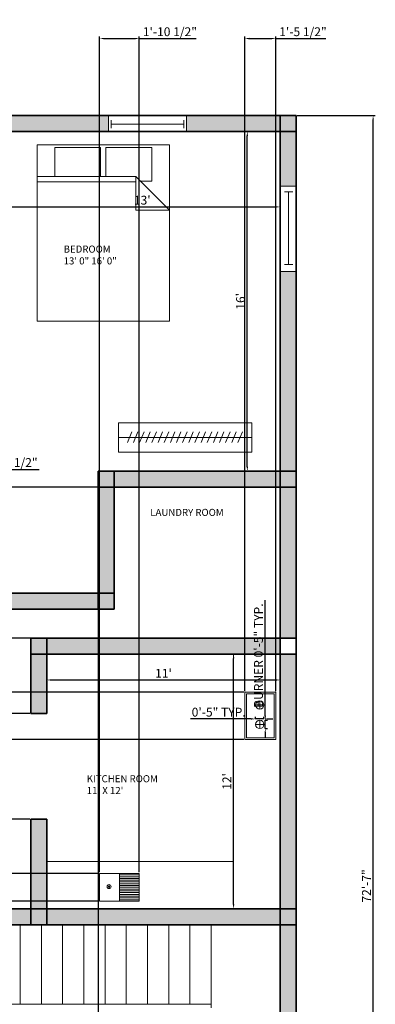
# Model space of a CAD drawing. Units: millimetres. Extents: x 2936 to 3516, y 349 to 1320.
# Tile 5 of 5: x 3315 to 3516, y 763 to 1320. Entities that reach past the tile are written whole.
import ezdxf

# ---------------------------------------------------------------- set-up
doc = ezdxf.new("R2010")
doc.units = ezdxf.units.MM
for name, color, linetype, lineweight in [('A-ANNO-DIMS', 3, 'Continuous', 13), ('A-AREA-IDEN', 190, 'Continuous', 18), ('A-EQPM', 140, 'Continuous', 18), ('A-FLOR-CASE', 140, 'Continuous', 18), ('A-FLOR-CASE-PATT', 140, 'Continuous', 13), ('A-FLOR-FIXT', 140, 'Continuous', 18), ('A-FLOR-FIXT-PATT', 140, 'Continuous', 13), ('A-WALL-PATT', 50, 'Continuous', 13), ('furniture', 140, 'Continuous', 18), ('staircase', 170, 'Continuous', 18), ('walls', 50, 'Continuous', 35), ('windows', 30, 'Continuous', 18)]:
    doc.layers.add(name, color=color, linetype=linetype, lineweight=lineweight)
doc.styles.get("Standard").update_dxf_attribs({"font": 'arial.ttf'})
doc.dimstyles.new('ISO-25', dxfattribs={"dimtxt": 5, "dimasz": 2.5, "dimexe": 1.25, "dimexo": 0.625, "dimtad": 1, "dimdec": 0, "dimlunit": 3, "dimtxsty": 'Standard', "dimcen": 2.5, "dimadec": 0, "dimazin": 0, "dimtfac": 1, "dimtdec": 0, "dimtmove": 0, "dimatfit": 3, "dimfxl": 1, "dimarcsym": 0})

# ---------------------------------------------------------------- blocks, each defined once
blk = doc.blocks.new('*U4')
for p, q in [((0, 4), (0, 0)), ((0, 2), (36, 2)), ((36, 4), (36, 0))]:
    blk.add_line(p, q)
blk = doc.blocks.new('Bed - Queen')
for p, q in [((0, -80.00003), (0, 0)), ((0, 0), (59.99999, 0)), ((59.99999, 0), (59.99999, -80.00003)), ((7.99999, -1.2), (28.79998, -1.2)), ((7.99999, -14.4), (7.99999, -1.2)), ((28.79998, -1.2), (28.79998, -14.4)), ((31.19999, -1.2), (51.99999, -1.2)), ((31.19999, -14.4), (31.19999, -1.2)), ((51.99999, -1.2), (51.99999, -16.4)), ((0, -14.4), (44.8, -14.4)), ((44.8, -16.8), (0, -16.8)), ((59.99999, -29.6), (44.8, -14.4)), ((44.8, -14.4), (44.8, -29.6)), ((51.99999, -16.4), (46.79936, -16.4)), ((44.8, -29.6), (59.99999, -29.6)), ((59.99999, -80.00003), (0, -80.00003))]:
    blk.add_line(p, q)
blk = doc.blocks.new('*D21')
at = {"layer": 'A-ANNO-DIMS', "color": 0, "lineweight": -2, "transparency": 16777216}
for p, q in [((3308.69, 1213.65), (3459.69, 1213.65)), ((3306.19, 1213.25), (3306.19, 1212.4)), ((3462.19, 1213.25), (3462.19, 1212.4))]:
    blk.add_line(p, q, dxfattribs=at)
at = {"layer": 'A-ANNO-DIMS', "color": 0, "transparency": 16777216}
for points in [[(3308.69, 1214.07), (3308.69, 1213.23), (3306.19, 1213.65)], [(3459.69, 1214.07), (3459.69, 1213.23), (3462.19, 1213.65)]]:
    blk.add_solid(points, dxfattribs=at)
at = {"layer": 'Defpoints', "color": 0, "transparency": 16777216}
for p in [(3306.19, 1213.88), (3462.19, 1213.88), (3462.19, 1213.65)]:
    blk.add_point(p, dxfattribs=at)
at = {"layer": 'A-ANNO-DIMS', "color": 0, "transparency": 16777216, "insert": (3384.19, 1216.83), "char_height": 5, "attachment_point": 5}
blk.add_mtext("13'", dxfattribs=at)
blk = doc.blocks.new('*D22')
at = {"layer": 'A-ANNO-DIMS', "color": 0, "lineweight": -2, "transparency": 16777216}
for p, q in [((3451.07, 1256.28), (3442.36, 1256.28)), ((3443.61, 1066.78), (3443.61, 1253.78)), ((3451.07, 1064.28), (3442.36, 1064.28))]:
    blk.add_line(p, q, dxfattribs=at)
at = {"layer": 'A-ANNO-DIMS', "color": 0, "transparency": 16777216}
for points in [[(3443.19, 1253.78), (3444.03, 1253.78), (3443.61, 1256.28)], [(3443.19, 1066.78), (3444.03, 1066.78), (3443.61, 1064.28)]]:
    blk.add_solid(points, dxfattribs=at)
at = {"layer": 'Defpoints', "color": 0, "transparency": 16777216}
for p in [(3443.61, 1256.28), (3451.7, 1256.28), (3451.7, 1064.28)]:
    blk.add_point(p, dxfattribs=at)
at = {"layer": 'A-ANNO-DIMS', "color": 0, "transparency": 16777216, "insert": (3440.43, 1160.28), "char_height": 5, "attachment_point": 5, "rotation": 90}
blk.add_mtext("16'", dxfattribs=at)
blk = doc.blocks.new('*D26')
at = {"layer": 'A-ANNO-DIMS', "color": 0, "lineweight": -2, "transparency": 16777216}
for p, q in [((3330.19, 947.94), (3330.19, 944.97)), ((3462.19, 947.94), (3462.19, 944.97)), ((3332.69, 946.22), (3459.69, 946.22))]:
    blk.add_line(p, q, dxfattribs=at)
at = {"layer": 'A-ANNO-DIMS', "color": 0, "transparency": 16777216}
for points in [[(3332.69, 946.64), (3332.69, 945.8), (3330.19, 946.22)], [(3459.69, 946.64), (3459.69, 945.8), (3462.19, 946.22)]]:
    blk.add_solid(points, dxfattribs=at)
at = {"layer": 'Defpoints', "color": 0, "transparency": 16777216}
for p in [(3330.19, 948.57), (3462.19, 948.57), (3462.19, 946.22)]:
    blk.add_point(p, dxfattribs=at)
at = {"layer": 'A-ANNO-DIMS', "color": 0, "transparency": 16777216, "insert": (3396.19, 949.36), "char_height": 5, "attachment_point": 5}
blk.add_mtext("11'", dxfattribs=at)
blk = doc.blocks.new('*D27')
at = {"layer": 'A-ANNO-DIMS', "color": 0, "lineweight": -2, "transparency": 16777216}
for p, q in [((3435.84, 819.36), (3435.84, 958.36)), ((3436.47, 960.86), (3437.09, 960.86)), ((3436.58, 816.86), (3434.59, 816.86))]:
    blk.add_line(p, q, dxfattribs=at)
at = {"layer": 'A-ANNO-DIMS', "color": 0, "transparency": 16777216}
for points in [[(3435.43, 958.36), (3436.26, 958.36), (3435.84, 960.86)], [(3435.43, 819.36), (3436.26, 819.36), (3435.84, 816.86)]]:
    blk.add_solid(points, dxfattribs=at)
at = {"layer": 'Defpoints', "color": 0, "transparency": 16777216}
for p in [(3435.84, 960.86), (3435.84, 960.86), (3437.21, 816.86)]:
    blk.add_point(p, dxfattribs=at)
at = {"layer": 'A-ANNO-DIMS', "color": 0, "transparency": 16777216, "insert": (3432.71, 888.86), "char_height": 5, "attachment_point": 5, "rotation": 90}
blk.add_mtext("12'", dxfattribs=at)
blk = doc.blocks.new('COOKTOP-BURNER')
for p, q in [((4.76, 2.38), (0, 2.38)), ((2.38, 4.76), (2.38, 0))]:
    blk.add_line(p, q)
blk.add_circle((2.38, 2.38), 2.38)
blk = doc.blocks.new('*D47')
at = {"layer": 'A-ANNO-DIMS', "color": 0, "lineweight": -2, "transparency": 16777216}
for p, q in [((3453.74, 925.98), (3453.74, 991.42)), ((3453.65, 923.48), (3454.99, 923.48)), ((3453.65, 918.72), (3454.99, 918.72)), ((3453.74, 918.72), (3453.74, 923.48)), ((3453.74, 916.22), (3453.74, 913.72))]:
    blk.add_line(p, q, dxfattribs=at)
at = {"layer": 'A-ANNO-DIMS', "color": 0, "transparency": 16777216}
for points in [[(3453.33, 925.98), (3454.16, 925.98), (3453.74, 923.48)], [(3453.33, 916.22), (3454.16, 916.22), (3453.74, 918.72)]]:
    blk.add_solid(points, dxfattribs=at)
at = {"layer": 'Defpoints', "color": 0, "transparency": 16777216}
for p in [(3453.03, 923.48), (3453.03, 918.72), (3453.74, 923.48)]:
    blk.add_point(p, dxfattribs=at)
at = {"layer": 'A-ANNO-DIMS', "color": 0, "transparency": 16777216, "insert": (3450.56, 959.95), "char_height": 5, "attachment_point": 5, "rotation": 90}
blk.add_mtext('BURNER 0\'-5" TYP.', dxfattribs=at)
blk = doc.blocks.new('*D48')
at = {"layer": 'A-ANNO-DIMS', "color": 0, "lineweight": -2, "transparency": 16777216}
for p, q in [((3445.77, 924.19), (3411.54, 924.19)), ((3448.27, 924.1), (3448.27, 925.44)), ((3453.03, 924.19), (3448.27, 924.19)), ((3453.03, 924.1), (3453.03, 925.44)), ((3455.53, 924.19), (3458.03, 924.19))]:
    blk.add_line(p, q, dxfattribs=at)
at = {"layer": 'A-ANNO-DIMS', "color": 0, "transparency": 16777216}
for points in [[(3445.77, 924.61), (3445.77, 923.78), (3448.27, 924.19)], [(3455.53, 924.61), (3455.53, 923.78), (3453.03, 924.19)]]:
    blk.add_solid(points, dxfattribs=at)
at = {"layer": 'Defpoints', "color": 0, "transparency": 16777216}
for p in [(3448.27, 924.19), (3448.27, 923.48), (3453.03, 923.48)]:
    blk.add_point(p, dxfattribs=at)
at = {"layer": 'A-ANNO-DIMS', "color": 0, "transparency": 16777216, "insert": (3427.41, 927.37), "char_height": 5, "attachment_point": 5}
blk.add_mtext('0\'-5" TYP.', dxfattribs=at)
blk = doc.blocks.new('*D53')
at = {"layer": 'A-ANNO-DIMS', "color": 0, "lineweight": -2, "transparency": 16777216}
for p, q in [((3228.24, 1071.35), (3228.24, 1064.03)), ((3272.91, 1071.35), (3272.91, 1064.03)), ((3230.74, 1065.28), (3270.41, 1065.28)), ((3272.91, 1065.28), (3325.8, 1065.28))]:
    blk.add_line(p, q, dxfattribs=at)
at = {"layer": 'A-ANNO-DIMS', "color": 0, "transparency": 16777216}
for points in [[(3230.74, 1065.69), (3230.74, 1064.86), (3228.24, 1065.28)], [(3270.41, 1065.69), (3270.41, 1064.86), (3272.91, 1065.28)]]:
    blk.add_solid(points, dxfattribs=at)
at = {"layer": 'Defpoints', "color": 0, "transparency": 16777216}
for p in [(3228.24, 1071.98), (3272.91, 1071.98), (3272.91, 1065.28)]:
    blk.add_point(p, dxfattribs=at)
at = {"layer": 'A-ANNO-DIMS', "color": 0, "transparency": 16777216, "insert": (3300.61, 1068.49), "char_height": 5, "attachment_point": 5}
blk.add_mtext('TABLE 3\'-8 1/2"', dxfattribs=at)
blk = doc.blocks.new('*D56')
at = {"layer": 'A-ANNO-DIMS', "color": 0, "lineweight": -2, "transparency": 16777216}
for p, q in [((3471.82, 1265.28), (3515.99, 1265.28)), ((3514.74, 396.79), (3514.74, 1262.78)), ((3471.82, 394.29), (3515.99, 394.29))]:
    blk.add_line(p, q, dxfattribs=at)
at = {"layer": 'A-ANNO-DIMS', "color": 0, "transparency": 16777216}
for points in [[(3514.33, 1262.78), (3515.16, 1262.78), (3514.74, 1265.28)], [(3514.33, 396.79), (3515.16, 396.79), (3514.74, 394.29)]]:
    blk.add_solid(points, dxfattribs=at)
at = {"layer": 'Defpoints', "color": 0, "transparency": 16777216}
for p in [(3471.19, 1265.28), (3514.74, 1265.28), (3471.19, 394.29)]:
    blk.add_point(p, dxfattribs=at)
at = {"layer": 'A-ANNO-DIMS', "color": 0, "transparency": 16777216, "insert": (3511.61, 829.78), "char_height": 5, "attachment_point": 5, "rotation": 90}
blk.add_mtext('72\'-7"', dxfattribs=at)
blk = doc.blocks.new('*D58')
at = {"layer": 'A-ANNO-DIMS', "color": 0, "lineweight": -2, "transparency": 16777216}
for p, q in [((3359.33, 1063.66), (3359.33, 349.48)), ((3471.19, 1063.66), (3471.19, 349.48)), ((3361.83, 350.73), (3468.69, 350.73))]:
    blk.add_line(p, q, dxfattribs=at)
at = {"layer": 'A-ANNO-DIMS', "color": 0, "transparency": 16777216}
for points in [[(3361.83, 351.15), (3361.83, 350.32), (3359.33, 350.73)], [(3468.69, 351.15), (3468.69, 350.32), (3471.19, 350.73)]]:
    blk.add_solid(points, dxfattribs=at)
at = {"layer": 'Defpoints', "color": 0, "transparency": 16777216}
for p in [(3359.33, 1064.28), (3471.19, 1064.28), (3471.19, 350.73)]:
    blk.add_point(p, dxfattribs=at)
at = {"layer": 'A-ANNO-DIMS', "color": 0, "transparency": 16777216, "insert": (3415.26, 353.91), "char_height": 5, "attachment_point": 5}
blk.add_mtext('9\'-4"', dxfattribs=at)
blk = doc.blocks.new('*D59')
at = {"layer": 'A-ANNO-DIMS', "color": 0, "lineweight": -2, "transparency": 16777216}
for p, q in [((3470.57, 1055.28), (2945.39, 1055.28)), ((2946.64, 972.36), (2946.64, 1052.78)), ((3470.57, 969.86), (2945.39, 969.86))]:
    blk.add_line(p, q, dxfattribs=at)
at = {"layer": 'A-ANNO-DIMS', "color": 0, "transparency": 16777216}
for points in [[(2946.22, 1052.78), (2947.06, 1052.78), (2946.64, 1055.28)], [(2946.22, 972.36), (2947.06, 972.36), (2946.64, 969.86)]]:
    blk.add_solid(points, dxfattribs=at)
at = {"layer": 'Defpoints', "color": 0, "transparency": 16777216}
for p in [(2946.64, 1055.28), (3471.19, 1055.28), (3471.19, 969.86)]:
    blk.add_point(p, dxfattribs=at)
at = {"layer": 'A-ANNO-DIMS', "color": 0, "transparency": 16777216, "insert": (2943.43, 1012.57), "char_height": 5, "attachment_point": 5, "rotation": 90}
blk.add_mtext('7\'-1 1/2"', dxfattribs=at)
blk = doc.blocks.new('*D60')
at = {"layer": 'A-ANNO-DIMS', "color": 0, "lineweight": -2, "transparency": 16777216}
for p, q in [((3320.57, 927.28), (2945.39, 927.28)), ((2946.64, 870.06), (2946.64, 924.78)), ((3320.57, 867.56), (2945.39, 867.56))]:
    blk.add_line(p, q, dxfattribs=at)
at = {"layer": 'A-ANNO-DIMS', "color": 0, "transparency": 16777216}
for points in [[(2946.22, 924.78), (2947.06, 924.78), (2946.64, 927.28)], [(2946.22, 870.06), (2947.06, 870.06), (2946.64, 867.56)]]:
    blk.add_solid(points, dxfattribs=at)
at = {"layer": 'Defpoints', "color": 0, "transparency": 16777216}
for p in [(2946.64, 927.28), (3321.19, 927.28), (3321.19, 867.56)]:
    blk.add_point(p, dxfattribs=at)
at = {"layer": 'A-ANNO-DIMS', "color": 0, "transparency": 16777216, "insert": (2943.43, 897.42), "char_height": 5, "attachment_point": 5, "rotation": 90}
blk.add_mtext('4\'-11 1/2"', dxfattribs=at)
blk = doc.blocks.new('*D61')
at = {"layer": 'A-ANNO-DIMS', "color": 0, "lineweight": -2, "transparency": 16777216}
for p, q in [((3360.06, 837.51), (3360.06, 1310.08)), ((3362.56, 1308.83), (3380.03, 1308.83)), ((3382.53, 837.51), (3382.53, 1310.08)), ((3382.53, 1308.83), (3414.63, 1308.83))]:
    blk.add_line(p, q, dxfattribs=at)
at = {"layer": 'A-ANNO-DIMS', "color": 0, "transparency": 16777216}
for points in [[(3362.56, 1309.25), (3362.56, 1308.42), (3360.06, 1308.83)], [(3380.03, 1309.25), (3380.03, 1308.42), (3382.53, 1308.83)]]:
    blk.add_solid(points, dxfattribs=at)
at = {"layer": 'Defpoints', "color": 0, "transparency": 16777216}
for p in [(3382.53, 1308.83), (3360.06, 836.89), (3382.53, 836.89)]:
    blk.add_point(p, dxfattribs=at)
at = {"layer": 'A-ANNO-DIMS', "color": 0, "transparency": 16777216, "insert": (3399.83, 1312.04), "char_height": 5, "attachment_point": 5}
blk.add_mtext('1\'-10 1/2"', dxfattribs=at)
blk = doc.blocks.new('*D62')
at = {"layer": 'A-ANNO-DIMS', "color": 0, "lineweight": -2, "transparency": 16777216}
for p, q in [((3359.43, 836.89), (2945.39, 836.89)), ((2946.64, 823.63), (2946.64, 834.39)), ((3359.43, 821.13), (2945.39, 821.13))]:
    blk.add_line(p, q, dxfattribs=at)
at = {"layer": 'A-ANNO-DIMS', "color": 0, "transparency": 16777216}
for points in [[(2946.22, 834.39), (2947.06, 834.39), (2946.64, 836.89)], [(2946.22, 823.63), (2947.06, 823.63), (2946.64, 821.13)]]:
    blk.add_solid(points, dxfattribs=at)
at = {"layer": 'Defpoints', "color": 0, "transparency": 16777216}
for p in [(2946.64, 836.89), (3360.06, 836.89), (3360.06, 821.13)]:
    blk.add_point(p, dxfattribs=at)
at = {"layer": 'A-ANNO-DIMS', "color": 0, "transparency": 16777216, "insert": (2943.51, 829.01), "char_height": 5, "attachment_point": 5, "rotation": 90}
blk.add_mtext('1\'-4"', dxfattribs=at)
blk = doc.blocks.new('*D63')
at = {"layer": 'A-ANNO-DIMS', "color": 0, "lineweight": -2, "transparency": 16777216}
for p, q in [((3442.16, 939.93), (3442.16, 1310.08)), ((3444.66, 1308.83), (3457.22, 1308.83)), ((3459.72, 939.93), (3459.72, 1310.08)), ((3459.72, 1308.83), (3487.95, 1308.83))]:
    blk.add_line(p, q, dxfattribs=at)
at = {"layer": 'A-ANNO-DIMS', "color": 0, "transparency": 16777216}
for points in [[(3444.66, 1309.25), (3444.66, 1308.42), (3442.16, 1308.83)], [(3457.22, 1309.25), (3457.22, 1308.42), (3459.72, 1308.83)]]:
    blk.add_solid(points, dxfattribs=at)
at = {"layer": 'Defpoints', "color": 0, "transparency": 16777216}
for p in [(3459.72, 1308.83), (3442.16, 939.3), (3459.72, 939.3)]:
    blk.add_point(p, dxfattribs=at)
at = {"layer": 'A-ANNO-DIMS', "color": 0, "transparency": 16777216, "insert": (3475.08, 1312.04), "char_height": 5, "attachment_point": 5}
blk.add_mtext('1\'-5 1/2"', dxfattribs=at)
blk = doc.blocks.new('*D64')
at = {"layer": 'A-ANNO-DIMS', "color": 0, "lineweight": -2, "transparency": 16777216}
for p, q in [((3441.54, 939.3), (2945.39, 939.3)), ((2946.64, 915.06), (2946.64, 936.8)), ((3441.54, 912.56), (2945.39, 912.56))]:
    blk.add_line(p, q, dxfattribs=at)
at = {"layer": 'A-ANNO-DIMS', "color": 0, "transparency": 16777216}
for points in [[(2946.22, 936.8), (2947.06, 936.8), (2946.64, 939.3)], [(2946.22, 915.06), (2947.06, 915.06), (2946.64, 912.56)]]:
    blk.add_solid(points, dxfattribs=at)
at = {"layer": 'Defpoints', "color": 0, "transparency": 16777216}
for p in [(2946.64, 939.3), (3442.16, 939.3), (3442.16, 912.56)]:
    blk.add_point(p, dxfattribs=at)
at = {"layer": 'A-ANNO-DIMS', "color": 0, "transparency": 16777216, "insert": (2943.43, 925.93), "char_height": 5, "attachment_point": 5, "rotation": 90}
blk.add_mtext('2\'-2 1/2"', dxfattribs=at)

msp = doc.modelspace()

# ---------------------------------------------------------------- hatches: boundary and pattern name
at = {"layer": 'A-FLOR-CASE-PATT'}
h = msp.add_hatch(dxfattribs=at)
h.set_pattern_fill('ANSI31', color=256, scale=1.008033, angle=22.079, style=0)
h.paths.add_polyline_path([(3374.29, 1080.42), (3440.31, 1080.42), (3442.84, 1086.41), (3376.82, 1086.41)])
at = {"layer": 'A-FLOR-FIXT-PATT'}
h = msp.add_hatch(dxfattribs=at)
h.set_pattern_fill('ANSI31', color=256, scale=0.314961, angle=-45, style=0)
h.paths.add_polyline_path([(3371.29, 821.89), (3382.53, 821.89), (3382.53, 836.89), (3371.29, 836.89)])
at = {"layer": 'A-WALL-PATT'}
h = msp.add_hatch(color=256, dxfattribs=at)
h.dxf.hatch_style = 1
h.paths.add_polyline_path([(2999.19, 1256.28), (2990.19, 1256.28), (2990.19, 1160.28), (2999.19, 1160.28)])
h.paths.add_polyline_path([(2999.19, 1265.28), (2990.19, 1265.28), (2990.19, 1256.28), (2999.19, 1256.28)])
h.paths.add_polyline_path([(3024.89, 1265.28), (2999.19, 1265.28), (2999.19, 1256.28), (3024.89, 1256.28)])
h.paths.add_polyline_path([(3074.24, 1160.28), (2999.19, 1160.28), (2999.19, 1151.28), (3072.14, 1151.28), (3072.14, 1152.43, -0.131652)])
h.paths.add_polyline_path([(2999.19, 1160.28), (2990.19, 1160.28), (2990.19, 1151.28), (2999.19, 1151.28)])
h.paths.add_polyline_path([(3123.19, 1256.28), (3114.19, 1256.28), (3114.19, 1160.28), (3123.19, 1160.28)])
h.paths.add_polyline_path([(3123.19, 1160.28), (3114.19, 1160.28), (3114.19, 1151.28), (3123.19, 1151.28)])
h.paths.add_polyline_path([(3114.19, 1160.28), (3087.85, 1160.28), (3087.85, 1152.43), (3087.85, 1151.28), (3114.19, 1151.28)])
h.paths.add_polyline_path([(3114.19, 1265.28), (3068.72, 1265.28), (3068.72, 1256.28), (3114.19, 1256.28)])
h.paths.add_polyline_path([(3123.19, 1265.28), (3114.19, 1265.28), (3114.19, 1256.28), (3123.19, 1256.28)])
h.paths.add_polyline_path([(3143.16, 1265.28), (3123.19, 1265.28), (3123.19, 1256.28), (3143.16, 1256.28)])
h.paths.add_polyline_path([(3214.19, 1265.28), (3187.49, 1265.28), (3187.49, 1256.28), (3214.19, 1256.28)])
h.paths.add_polyline_path([(3214.19, 1160.28), (3140.09, 1160.28, -0.121149), (3141.88, 1153), (3141.88, 1151.28), (3214.19, 1151.28)])
h.paths.add_polyline_path([(3223.19, 1256.28), (3214.19, 1256.28), (3214.19, 1160.28), (3223.19, 1160.28)])
h.paths.add_polyline_path([(3223.19, 1160.28), (3214.19, 1160.28), (3214.19, 1151.28), (3223.19, 1151.28)])
h.paths.add_polyline_path([(3223.19, 1151.28), (3214.19, 1151.28), (3214.19, 1134.28), (3223.19, 1134.28)])
h.paths.add_polyline_path([(3223.19, 1134.28), (3214.19, 1134.28), (3214.19, 1125.28), (3223.19, 1125.28)])
h.paths.add_polyline_path([(3223.19, 1125.28), (3214.19, 1125.28), (3214.19, 1064.28), (3223.19, 1064.28)])
h.paths.add_polyline_path([(3281.06, 1126.52, -0.130008), (3283.12, 1134.28), (3223.19, 1134.28), (3223.19, 1125.28), (3281.06, 1125.28)])
h.paths.add_polyline_path([(3223.19, 1265.28), (3214.19, 1265.28), (3214.19, 1256.28), (3223.19, 1256.28)])
h.paths.add_polyline_path([(3235.61, 1265.28), (3223.19, 1265.28), (3223.19, 1256.28), (3235.61, 1256.28)])
h.paths.add_polyline_path([(3297.19, 1265.28), (3278.85, 1265.28), (3278.85, 1256.28), (3297.19, 1256.28)])
h.paths.add_polyline_path([(3306.19, 1265.28), (3297.19, 1265.28), (3297.19, 1256.28), (3306.19, 1256.28)])
h.paths.add_polyline_path([(3306.19, 1256.28), (3297.19, 1256.28), (3297.19, 1134.28), (3306.19, 1134.28)])
h.paths.add_polyline_path([(3306.19, 1134.28), (3297.19, 1134.28), (3297.19, 1125.28), (3306.19, 1125.28)])
h.paths.add_polyline_path([(3306.19, 1125.28), (3297.19, 1125.28), (3297.19, 1084.87), (3305.61, 1084.87), (3306.19, 1084.87)])
h.paths.add_polyline_path([(3365.17, 1265.28), (3306.19, 1265.28), (3306.19, 1256.28), (3365.17, 1256.28)])
h.paths.add_polyline_path([(3462.19, 1265.28), (3409.24, 1265.28), (3409.24, 1256.28), (3462.19, 1256.28)])
h.paths.add_polyline_path([(3471.19, 1265.28), (3462.19, 1265.28), (3462.19, 1256.28), (3471.19, 1256.28)])
h.paths.add_polyline_path([(3471.19, 1256.28), (3462.19, 1256.28), (3462.19, 1225.41), (3471.19, 1225.41)])
h.paths.add_polyline_path([(3471.19, 1177.19), (3462.19, 1177.19), (3462.19, 1064.28), (3471.19, 1064.28)])
h.paths.add_polyline_path([(3462.19, 1064.28), (3368.33, 1064.28), (3368.33, 1055.28), (3462.19, 1055.28)])
h.paths.add_polyline_path([(3471.19, 1064.28), (3462.19, 1064.28), (3462.19, 1055.28), (3471.19, 1055.28)])
h.paths.add_polyline_path([(3471.19, 1055.28), (3462.19, 1055.28), (3462.19, 969.86), (3471.19, 969.86)])
h.paths.add_polyline_path([(3368.33, 1055.28), (3359.33, 1055.28), (3359.33, 995.28), (3368.33, 995.28)])
h.paths.add_polyline_path([(3368.33, 1064.28), (3359.33, 1064.28), (3359.33, 1055.28), (3368.33, 1055.28)])
h.paths.add_polyline_path([(3359.33, 995.28), (3306.19, 995.28), (3306.19, 986.28), (3359.33, 986.28)])
h.paths.add_polyline_path([(3368.33, 995.28), (3359.33, 995.28), (3359.33, 986.28), (3368.33, 986.28)])
h.paths.add_polyline_path([(3306.19, 995.28), (3297.19, 995.28), (3297.19, 986.28), (3306.19, 986.28)])
h.paths.add_polyline_path([(3306.19, 1011.04), (3298.85, 1011.04), (3297.19, 1011.04), (3297.19, 995.28), (3306.19, 995.28)])
h.paths.add_polyline_path([(3306.19, 1055.28), (3297.19, 1055.28), (3297.19, 1026.75), (3298.85, 1026.75, -0.122211), (3306.19, 1024.93)])
h.paths.add_polyline_path([(3306.19, 1064.28), (3297.19, 1064.28), (3297.19, 1055.28), (3306.19, 1055.28)])
h.paths.add_polyline_path([(3297.19, 1064.28), (3223.19, 1064.28), (3223.19, 1055.28), (3297.19, 1055.28)])
h.paths.add_polyline_path([(3223.19, 1064.28), (3214.19, 1064.28), (3214.19, 1055.28), (3223.19, 1055.28)])
h.paths.add_polyline_path([(3223.19, 1055.28), (3214.19, 1055.28), (3214.19, 1031.96), (3221.18, 1031.96), (3223.19, 1031.96)])
h.paths.add_polyline_path([(3223.19, 1016.25), (3221.18, 1016.25, -0.11578), (3214.19, 1017.89), (3214.19, 995.28), (3223.19, 995.28)])
h.paths.add_polyline_path([(3223.19, 995.28), (3214.19, 995.28), (3214.19, 986.28), (3223.19, 986.28)])
h.paths.add_polyline_path([(3214.19, 995.28), (3061.3, 995.28), (3061.3, 986.28), (3214.19, 986.28)])
h.paths.add_polyline_path([(2999.19, 1151.28), (2990.19, 1151.28), (2990.19, 995.28), (2999.19, 995.28)])
h.paths.add_polyline_path([(2999.19, 986.28), (2990.19, 986.28), (2990.19, 816.86), (2999.19, 816.86)])
h.paths.add_polyline_path([(2999.19, 995.28), (2990.19, 995.28), (2990.19, 986.28), (2999.19, 986.28)])
h.paths.add_polyline_path([(3016.23, 995.28), (2999.19, 995.28), (2999.19, 986.28), (3016.23, 986.28)])
h.paths.add_polyline_path([(2999.19, 807.86), (2990.19, 807.86), (2990.19, 683.86), (2999.19, 683.86)])
h.paths.add_polyline_path([(2999.19, 816.86), (2990.19, 816.86), (2990.19, 807.86), (2999.19, 807.86)])
h.paths.add_polyline_path([(3179.19, 816.86), (2999.19, 816.86), (2999.19, 807.86), (3179.19, 807.86)])
h.paths.add_polyline_path([(3188.19, 780.83), (3187.16, 780.83, -0.133677), (3179.19, 783), (3179.19, 683.86), (3188.19, 683.86)])
h.paths.add_polyline_path([(3188.19, 807.86), (3179.19, 807.86), (3179.19, 796.54), (3187.16, 796.54), (3188.19, 796.54)])
h.paths.add_polyline_path([(3188.19, 816.86), (3179.19, 816.86), (3179.19, 807.86), (3188.19, 807.86)])
h.paths.add_polyline_path([(3196.08, 816.86), (3188.19, 816.86), (3188.19, 807.86), (3196.08, 807.86)])
h.paths.add_polyline_path([(3321.19, 816.86), (3227.5, 816.86), (3227.5, 807.86), (3321.19, 807.86)])
h.paths.add_polyline_path([(3330.19, 867.56), (3321.19, 867.56), (3321.19, 816.86), (3330.19, 816.86)])
h.paths.add_polyline_path([(3330.19, 816.86), (3321.19, 816.86), (3321.19, 807.86), (3330.19, 807.86)])
h.paths.add_polyline_path([(3462.19, 816.86), (3330.19, 816.86), (3330.19, 807.86), (3462.19, 807.86)])
h.paths.add_polyline_path([(3471.19, 960.86), (3462.19, 960.86), (3462.19, 816.86), (3471.19, 816.86)])
h.paths.add_polyline_path([(3471.19, 816.86), (3462.19, 816.86), (3462.19, 807.86), (3471.19, 807.86)])
h.paths.add_polyline_path([(3471.19, 807.86), (3462.19, 807.86), (3462.19, 394.29), (3471.19, 394.29)])
h.paths.add_polyline_path([(3462.19, 715.94), (3227.5, 715.94), (3227.5, 708.13), (3227.5, 706.94), (3462.19, 706.94)])
h.paths.add_polyline_path([(3196.08, 715.94), (3188.19, 715.94), (3188.19, 706.94), (3196.08, 706.94), (3196.08, 708.13)])
h.paths.add_polyline_path([(2999.19, 674.86), (2990.19, 674.86), (2990.19, 554.86), (2999.19, 554.86)])
h.paths.add_polyline_path([(3179.19, 683.86), (2999.19, 683.86), (2999.19, 674.86), (3179.19, 674.86)])
h.paths.add_polyline_path([(2999.19, 683.86), (2990.19, 683.86), (2990.19, 674.86), (2999.19, 674.86)])
h.paths.add_polyline_path([(2999.19, 545.86), (2990.19, 545.86), (2990.19, 394.29), (2999.19, 394.29)])
h.paths.add_polyline_path([(3047.58, 554.86), (2999.19, 554.86), (2999.19, 545.86), (3047.58, 545.86)])
h.paths.add_polyline_path([(2999.19, 554.86), (2990.19, 554.86), (2990.19, 545.86), (2999.19, 545.86)])
h.paths.add_polyline_path([(3179.19, 554.86), (3096.19, 554.86), (3096.19, 545.86), (3179.19, 545.86)])
h.paths.add_polyline_path([(3188.19, 554.86), (3179.19, 554.86), (3179.19, 545.86), (3188.19, 545.86)])
h.paths.add_polyline_path([(3188.19, 652.99), (3187.11, 652.99, -0.132871), (3179.19, 655.13), (3179.19, 554.86), (3188.19, 554.86)])
h.paths.add_polyline_path([(3188.19, 683.86), (3179.19, 683.86), (3179.19, 674.86), (3188.19, 674.86)])
h.paths.add_polyline_path([(3188.19, 674.86), (3179.19, 674.86), (3179.19, 668.7), (3187.11, 668.7), (3188.19, 668.7)])
h.paths.add_polyline_path([(3462.19, 969.86), (3330.19, 969.86), (3330.19, 960.86), (3462.19, 960.86)])
h.paths.add_polyline_path([(3330.19, 969.86), (3321.19, 969.86), (3321.19, 960.86), (3330.19, 960.86)])
h.paths.add_polyline_path([(3330.19, 960.86), (3321.19, 960.86), (3321.19, 927.28), (3330.19, 927.28)])

# ---------------------------------------------------------------- linework, layer by layer
at = {"layer": 'A-EQPM'}
for points in [[(3442.16, 939.3), (3459.72, 939.3), (3459.72, 912.56), (3442.16, 912.56)], [(3443.16, 938.3), (3458.72, 938.3), (3458.72, 913.56), (3443.16, 913.56)]]:
    msp.add_lwpolyline(points, close=True, dxfattribs=at)
at = {"layer": 'A-FLOR-CASE'}
for p, q in [((3446.25, 1083.32), (3370.75, 1083.32)), ((3462.19, 960.86), (3435.84, 960.86)), ((3435.84, 960.86), (3435.84, 843.53)), ((3435.84, 843.53), (3330.19, 843.53))]:
    msp.add_line(p, q, dxfattribs=at)
msp.add_lwpolyline([(3370.75, 1075.05), (3446.25, 1075.05), (3446.25, 1091.59), (3370.75, 1091.59)], close=True, dxfattribs=at)
at = {"layer": 'A-FLOR-FIXT'}
msp.add_line((3371.29, 821.13), (3371.29, 836.89), dxfattribs=at)
msp.add_lwpolyline([(3360.06, 836.89), (3382.53, 836.89), (3382.53, 821.13), (3360.06, 821.13)], close=True, dxfattribs=at)
for radius in [1.13, 0.415]:
    msp.add_circle((3365.43, 829.39), radius, dxfattribs=at)
at = {"layer": 'staircase'}
for p, q in [((3315.17, 807.86), (3315.17, 762.86)), ((3327.17, 807.86), (3327.17, 762.86)), ((3339.17, 807.86), (3339.17, 762.86)), ((3351.17, 807.86), (3351.17, 762.86)), ((3363.17, 807.86), (3363.17, 762.86)), ((3375.17, 807.86), (3375.17, 762.86)), ((3387.17, 807.86), (3387.17, 762.86)), ((3399.17, 807.86), (3399.17, 762.86)), ((3411.17, 807.86), (3411.17, 762.86)), ((3423.17, 807.86), (3423.17, 762.86)), ((3423.17, 762.86), (3255.17, 762.86)), ((3423.17, 760.86), (3423.17, 762.86))]:
    msp.add_line(p, q, dxfattribs=at)
at = {"layer": 'walls'}
for p, q in [((2990.19, 1265.28), (3471.19, 1265.28)), ((3462.19, 1265.28), (3462.19, 394.29)), ((3471.19, 1265.28), (3471.19, 394.29)), ((2990.19, 1256.28), (3471.19, 1256.28)), ((3359.33, 986.28), (3359.33, 1064.28)), ((3359.33, 1064.28), (3471.19, 1064.28)), ((3368.33, 986.28), (3368.33, 1064.28)), ((3359.33, 1055.28), (3471.19, 1055.28)), ((3297.19, 995.28), (3368.33, 995.28)), ((3297.19, 986.28), (3368.33, 986.28)), ((3471.19, 969.86), (3321.19, 969.86)), ((3321.19, 969.86), (3321.19, 927.28)), ((3330.19, 969.86), (3330.19, 927.28)), ((3471.19, 960.86), (3321.19, 960.86)), ((3321.19, 927.28), (3330.19, 927.28)), ((3321.19, 867.56), (3330.19, 867.56)), ((3321.19, 867.56), (3321.19, 807.86)), ((3330.19, 867.56), (3330.19, 807.86)), ((3471.19, 816.86), (3226.81, 816.86)), ((3471.19, 807.86), (3226.81, 807.86))]:
    msp.add_line(p, q, dxfattribs=at)
at = {"layer": 'windows'}
for p, q in [((3365.17, 1265.28), (3365.17, 1256.28)), ((3409.24, 1265.28), (3409.24, 1256.28)), ((3471.19, 1225.41), (3462.19, 1225.41)), ((3471.19, 1177.19), (3462.19, 1177.19))]:
    msp.add_line(p, q, dxfattribs=at)

# ---------------------------------------------------------------- block references
at = {"layer": 'A-EQPM'}
msp.add_blockref('COOKTOP-BURNER', (3448.27, 929.69), dxfattribs=at)
at = {"layer": 'A-EQPM', "rotation": 90.00000000001096}
msp.add_blockref('COOKTOP-BURNER', (3453.03, 918.72), dxfattribs=at)
at = {"layer": 'furniture', "xscale": 1.245124643961403, "yscale": 1.245124643961403, "zscale": 1.245124643961403}
msp.add_blockref('Bed - Queen', (3324.8, 1248.69), dxfattribs=at)
at = {"layer": 'windows', "xscale": 1.142279500402185, "yscale": 1.142279500402185, "zscale": 1.142279500402185}
msp.add_blockref('*U4', (3366.6, 1258.21), dxfattribs=at)
at = {"layer": 'windows', "xscale": 1.142279500402185, "yscale": 1.142279500402185, "zscale": 1.142279500402185, "rotation": 270}
msp.add_blockref('*U4', (3464.69, 1222.17), dxfattribs=at)

# ---------------------------------------------------------------- texts
at = {"layer": 'A-AREA-IDEN', "char_height": 4, "attachment_point": 1}
for s, width, insert in [('BEDROOM \\P13\' 0" 16\' 0"', 48.3973, (3339.73, 1191.81)), ('LAUNDRY ROOM', 52.0724, (3388.72, 1042.95)), ("KITCHEN ROOM \\P11' X 12'", 72.3742, (3352.78, 892.39))]:
    msp.add_mtext_dynamic_manual_height_columns(s, width=width, gutter_width=12.5, heights=[0], dxfattribs=dict(at, insert=insert))

# ---------------------------------------------------------------- dimensions: what is measured, and where the dimension line sits
at = {"layer": 'A-ANNO-DIMS'}
for base, p1, p2, override, picture, middle in [((3382.53, 1308.83), (3360.06, 836.89), (3382.53, 836.89), {"dimdec": 1, "dimlfac": 1, "dimrnd": 0, "dimzin": 1, "dimdsep": 46, "dimlunit": 4, "dimfrac": 2}, '*D61', (3399.83, 1312.04)), ((3459.72, 1308.83), (3442.16, 939.3), (3459.72, 939.3), {"dimdec": 1, "dimlfac": 1, "dimrnd": 0, "dimzin": 1, "dimdsep": 46, "dimlunit": 4, "dimfrac": 2}, '*D63', (3475.08, 1312.04)), ((3462.19, 1213.65), (3306.19, 1213.88), (3462.19, 1213.88), {"dimclrd": 0, "dimclre": 0, "dimclrt": 0}, '*D21', (3384.19, 1216.83)), ((3471.19, 350.73), (3359.33, 1064.28), (3471.19, 1064.28), {"dimdec": 1, "dimlfac": 1, "dimrnd": 0, "dimzin": 1, "dimdsep": 46, "dimlunit": 4, "dimfrac": 2}, '*D58', (3415.26, 353.91)), ((3462.19, 946.22), (3330.19, 948.57), (3462.19, 948.57), {"dimclrd": 0, "dimclre": 0, "dimclrt": 0}, '*D26', (3396.19, 949.36))]:
    dim = msp.add_linear_dim(base=base, p1=p1, p2=p2, dimstyle='ISO-25', override=override, dxfattribs=at)
    dim.commit()
    dim.dimension.update_dxf_attribs({"geometry": picture, "text_midpoint": middle})
for base, p1, p2, override, picture, middle in [((3514.74, 1265.28), (3471.19, 394.29), (3471.19, 1265.28), {"dimdec": 1, "dimlfac": 1, "dimrnd": 0, "dimzin": 1, "dimdsep": 46, "dimlunit": 4, "dimfrac": 2}, '*D56', (3511.61, 829.78)), ((3443.61, 1256.28), (3451.7, 1064.28), (3451.7, 1256.28), {"dimclrd": 0, "dimclre": 0, "dimclrt": 0}, '*D22', (3440.43, 1160.28)), ((2946.64, 1055.28), (3471.19, 969.86), (3471.19, 1055.28), {"dimdec": 1, "dimlfac": 1, "dimrnd": 0, "dimzin": 1, "dimdsep": 46, "dimlunit": 4, "dimfrac": 2}, '*D59', (2943.43, 1012.57)), ((3435.84, 960.86), (3437.21, 816.86), (3435.84, 960.86), {"dimclrd": 0, "dimclre": 0, "dimclrt": 0}, '*D27', (3432.71, 888.86)), ((2946.64, 939.3), (3442.16, 912.56), (3442.16, 939.3), {"dimdec": 1, "dimlfac": 1, "dimrnd": 0, "dimzin": 1, "dimdsep": 46, "dimlunit": 4, "dimfrac": 2}, '*D64', (2943.43, 925.93)), ((2946.64, 927.28), (3321.19, 867.56), (3321.19, 927.28), {"dimdec": 1, "dimlfac": 1, "dimrnd": 0, "dimzin": 1, "dimdsep": 46, "dimlunit": 4, "dimfrac": 2}, '*D60', (2943.43, 897.42)), ((2946.64, 836.89), (3360.06, 821.13), (3360.06, 836.89), {"dimdec": 1, "dimlfac": 1, "dimrnd": 0, "dimzin": 1, "dimdsep": 46, "dimlunit": 4, "dimfrac": 2}, '*D62', (2943.51, 829.01))]:
    dim = msp.add_linear_dim(base=base, p1=p1, p2=p2, angle=90, dimstyle='ISO-25', override=override, dxfattribs=at)
    dim.commit()
    dim.dimension.update_dxf_attribs({"geometry": picture, "text_midpoint": middle})
dim = msp.add_linear_dim(base=(3272.91, 1065.28), p1=(3228.24, 1071.98), p2=(3272.91, 1071.98), text='TABLE <>', dimstyle='ISO-25', override={"dimdec": 1, "dimlfac": 1, "dimrnd": 0, "dimzin": 1, "dimdsep": 46, "dimlunit": 4, "dimfrac": 2}, dxfattribs=at)
dim.commit()
dim.dimension.update_dxf_attribs({"geometry": '*D53', "text_midpoint": (3300.61, 1068.49)})
for base, p1, p2, angle, text, picture, middle in [((3453.74, 923.48), (3453.03, 918.72), (3453.03, 923.48), 90, 'BURNER <> TYP.', '*D47', (3450.56, 959.95)), ((3448.27, 924.19), (3453.03, 923.48), (3448.27, 923.48), 180, '<> TYP.', '*D48', (3427.41, 927.37))]:
    dim = msp.add_linear_dim(base=base, p1=p1, p2=p2, angle=angle, text=text, dimstyle='ISO-25', override={"dimdec": 1, "dimlfac": 1, "dimrnd": 0, "dimzin": 1, "dimdsep": 46, "dimlunit": 4, "dimfrac": 2}, dxfattribs=at)
    dim.commit()
    dim.dimension.update_dxf_attribs({"geometry": picture, "text_midpoint": middle})

doc.saveas('drawing.dxf')
